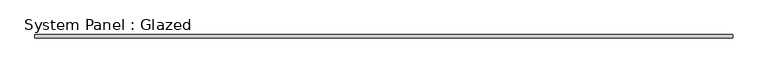
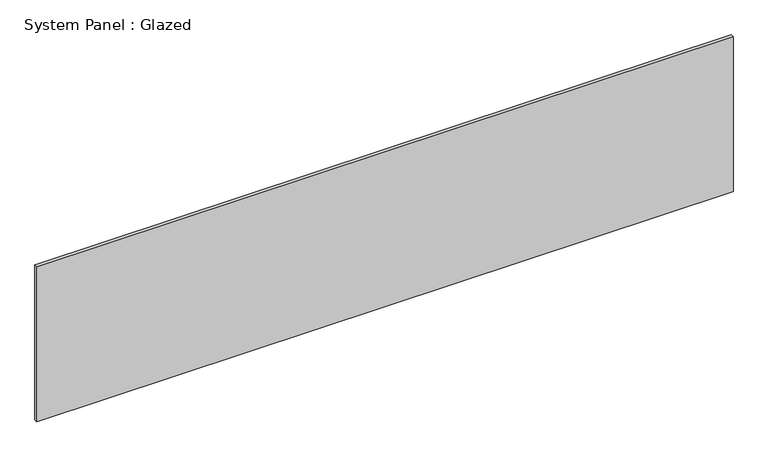
"""IFC4 building model written with IfcOpenShell, lengths in millimetres: plate geometry, System Panel : Glazed."""

from ifc_helpers import new_model, si_unit, origin, origin_with_axes, place, context, project, spatial, polyline, outline, extrude, source, transform, mapped, element, save


def system_panel_glazed_cbf88504(model_context):
    return source(origin(), model_context, "Body", "SweptSolid", [
        extrude(outline(polyline([(2590.0990733, 19.05), (-2590.0990733, 19.05), (-2590.0990733, 44.45), (2590.0990733, 44.45), (2590.0990733, 19.05)])), origin_with_axes(), (0.0, 0.0, 1.0), 1219.2),
    ])


if __name__ == "__main__":
    model = new_model("IFC4")
    model_context = context("Model", 3, world=origin())
    ifc_project = project(units=[si_unit("LENGTHUNIT", "METRE", prefix="MILLI")], contexts=[model_context])
    site = spatial("IfcSite", under=ifc_project)
    building = spatial("IfcBuilding", under=site)
    placement = place(None, origin())
    system_panel_glazed_shape = system_panel_glazed_cbf88504(model_context)
    element("IfcPlate", 1, ObjectType="System Panel : Glazed", at=placement, inside=building, context=model_context, shape_type="MappedRepresentation", body=[
        mapped(system_panel_glazed_shape, transform((0.0, 0.0, 0.0), x_axis=(1.0, 0.0, 0.0), y_axis=(0.0, 1.0, 0.0), z_axis=(0.0, 0.0, 1.0))),
    ])
    save(model, "model.ifc")

# Revit data of these elements
# Type "System Panel : Glazed"
#   Construction Type Id = "GSP4R"
#   Analytic Construction = "1/8 in Pilkington single glazing"
#   Visual Light Transmittance = 0.9
#   Solar Heat Gain Coefficient = 0.86
#   Heat Transfer Coefficient (U) = 1.18115 BTU/(h·ft²·°F)
# Element 1 (IfcPlate, "System Panel : Glazed")
#   Materials on its faces: "Glass"
# Materials
#   "Glass": class "Glass", colour RGB 0 128 192, transparency 0.75, Description = "Soda Lime Glass", Cost = 0
